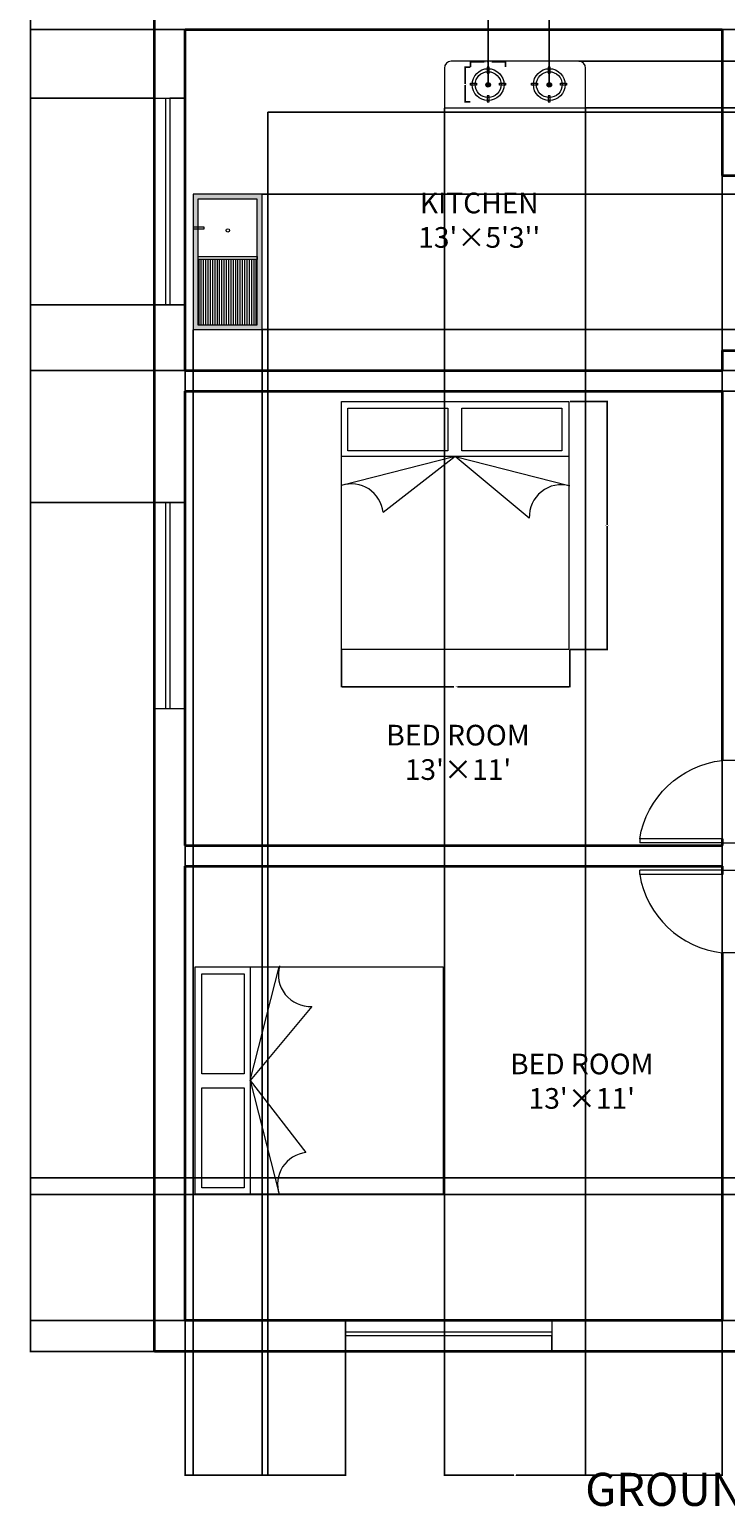
# Model space of a CAD drawing. Units: inches. Extents: x 1108 to 1543, y 442 to 1097.
# Tile 1 of 3: x 1108 to 1310, y 442 to 871. Entities that reach past the tile are written whole.
import ezdxf

# ---------------------------------------------------------------- set-up
doc = ezdxf.new("R2010")
doc.units = ezdxf.units.IN
for name, color, linetype, lineweight in [('A-ANNO-DIMS', 2, 'Continuous', 18), ('A-ANNO-TEXT', 7, 'Continuous', 25), ('A-AREA-IDEN', 7, 'Continuous', 18), ('A-DOOR', 4, 'Continuous', 18), ('A-EQPM', 8, 'Continuous', 18), ('A-FLOR-CASE', 8, 'Continuous', 25), ('A-FLOR-FIXT', 9, 'Continuous', 18), ('A-FLOR-FIXT-PATT', 9, 'Continuous', 13), ('A-FURN', 8, 'Continuous', 18), ('A-GLAZ', 5, 'Continuous', 18), ('A-WALL', 7, 'Continuous', 35)]:
    doc.layers.add(name, color=color, linetype=linetype, lineweight=lineweight)
doc.styles.get("Standard").update_dxf_attribs({"font": 'times.ttf'})
doc.dimstyles.get("Standard").update_dxf_attribs({"dimtxt": 0.18, "dimasz": 0.18, "dimexe": 0.18, "dimexo": 0.0625, "dimgap": 0.09, "dimtad": 0, "dimtih": 1, "dimtoh": 1, "dimdec": 4, "dimzin": 0, "dimdsep": 46, "dimtxsty": 'Standard', "dimcen": 0.09, "dimadec": 0, "dimazin": 0, "dimtfac": 1, "dimtdec": 4, "dimtofl": 0, "dimtmove": 0, "dimatfit": 3, "dimfxl": 1, "dimtolj": 1, "dimtzin": 0, "dimarcsym": 0})

# ---------------------------------------------------------------- blocks, each defined once
blk = doc.blocks.new('d')
for p, q in [((1309.33, 626.48), (1285.33, 626.48)), ((1285.33, 625.28), (1285.33, 626.48)), ((1309.33, 626.48), (1315.33, 626.48)), ((1309.33, 625.28), (1285.33, 625.28)), ((1315.33, 602.48), (1309.33, 602.48))]:
    blk.add_line(p, q)
blk.add_arc((1312.52, 629.86), 27.57, 189.5705, 263.3671)
blk = doc.blocks.new('BED-DOUBLE-66X72')
for p, q in [((0, 0), (0, 72)), ((0, 72), (66, 72)), ((66, 72), (66, 0)), ((66, 56.1), (0, 56.1)), ((33, 56.1), (0, 47.62)), ((33, 56.1), (12.08, 39.84)), ((33, 56.1), (66, 47.62)), ((54.54, 38.14), (33, 56.1)), ((66, 0), (0, 0))]:
    blk.add_line(p, q)
for points in [[(30.92, 70.13), (30.92, 57.75), (1.83, 57.75), (1.83, 70.13)], [(64.01, 70.13), (64.01, 57.75), (34.92, 57.75), (34.92, 70.13)]]:
    blk.add_lwpolyline(points, close=True)
for centre, radius, start, end in [((2.92, 38.89), 9.21, 5.9499, 108.4921), ((63.85, 38.55), 9.32, 74.4856, 182.5542)]:
    blk.add_arc(centre, radius, start, end)
blk = doc.blocks.new('WIN-60IN')
for p, q in [((-9, -60), (-9, 0)), ((-9, 0), (0, 0)), ((-5.7, -60), (-5.7, 0)), ((0, 0), (-4.5, 0)), ((-4.5, 0), (-4.5, -60)), ((0, 0), (0, -60)), ((0, -60), (-9, -60)), ((-4.5, -60), (-5.7, -60))]:
    blk.add_line(p, q)
blk = doc.blocks.new('HOB-BURNER')
h = blk.add_hatch(color=256)
h.dxf.hatch_style = 1
h.paths.add_polyline_path([(0.67, -0.05, 1), (-0.65, -0.05, 1)])
for points in [[(-0.28, 3.35), (0.3, 3.35), (0.3, 5.06), (-0.28, 5.06)], [(-5.14, 0.42), (-3.39, 0.42), (-3.39, -0.14), (-5.14, -0.14)], [(3.29, 0.42), (5.04, 0.42), (5.04, -0.14), (3.29, -0.14)], [(-0.28, -5), (0.3, -5), (0.3, -3.29), (-0.28, -3.29)]]:
    blk.add_lwpolyline(points, close=True)
for centre, radius in [((0, 0), 4.63), ((0, 0), 3.76), ((0.01, -0.05), 0.661)]:
    blk.add_circle(centre, radius)
blk = doc.blocks.new('*D11')
at = {"layer": 'A-ANNO-DIMS', "color": 0, "lineweight": -2, "transparency": 16777216}
for p, q in [((1265.13, 762.59), (1276.05, 762.59)), ((1275.87, 762.41), (1275.87, 726.77)), ((1275.87, 690.77), (1275.87, 726.41)), ((1265.13, 690.59), (1276.05, 690.59))]:
    blk.add_line(p, q, dxfattribs=at)
at = {"layer": 'A-ANNO-DIMS', "color": 0, "transparency": 16777216}
for points in [[(1275.84, 762.41), (1275.9, 762.41), (1275.87, 762.59)], [(1275.84, 690.77), (1275.9, 690.77), (1275.87, 690.59)]]:
    blk.add_solid(points, dxfattribs=at)
at = {"layer": 'Defpoints', "color": 0, "transparency": 16777216}
for p in [(1265.07, 762.59), (1275.87, 762.59), (1265.07, 690.59)]:
    blk.add_point(p, dxfattribs=at)
at = {"layer": 'A-ANNO-DIMS', "color": 0, "transparency": 16777216, "insert": (1275.87, 726.59), "char_height": 0.18, "attachment_point": 5}
blk.add_mtext('\\A1;BED 72 TYP.', dxfattribs=at)
blk = doc.blocks.new('*D12')
at = {"layer": 'A-ANNO-DIMS', "color": 0, "lineweight": -2, "transparency": 16777216}
for p, q in [((1198.72, 690.53), (1198.72, 679.61)), ((1265.07, 690.53), (1265.07, 679.61)), ((1198.9, 679.79), (1231.37, 679.79)), ((1264.89, 679.79), (1232.42, 679.79))]:
    blk.add_line(p, q, dxfattribs=at)
at = {"layer": 'A-ANNO-DIMS', "color": 0, "transparency": 16777216}
for points in [[(1198.9, 679.82), (1198.9, 679.76), (1198.72, 679.79)], [(1264.89, 679.82), (1264.89, 679.76), (1265.07, 679.79)]]:
    blk.add_solid(points, dxfattribs=at)
at = {"layer": 'Defpoints', "color": 0, "transparency": 16777216}
for p in [(1198.72, 690.59), (1265.07, 690.59), (1265.07, 679.79)]:
    blk.add_point(p, dxfattribs=at)
at = {"layer": 'A-ANNO-DIMS', "color": 0, "transparency": 16777216, "insert": (1231.89, 679.79), "char_height": 0.18, "attachment_point": 5}
blk.add_mtext('\\A1;66 TYP.', dxfattribs=at)
blk = doc.blocks.new('*D13')
at = {"layer": 'A-ANNO-DIMS', "color": 0, "lineweight": -2, "transparency": 16777216}
for p, q in [((1236.15, 859.8), (1236.15, 861.45)), ((1236.33, 861.27), (1240.14, 861.27)), ((1246.15, 861.27), (1242.34, 861.27)), ((1246.33, 859.8), (1246.33, 861.45))]:
    blk.add_line(p, q, dxfattribs=at)
at = {"layer": 'A-ANNO-DIMS', "color": 0, "transparency": 16777216}
for points in [[(1236.33, 861.3), (1236.33, 861.24), (1236.15, 861.27)], [(1246.15, 861.3), (1246.15, 861.24), (1246.33, 861.27)]]:
    blk.add_solid(points, dxfattribs=at)
at = {"layer": 'Defpoints', "color": 0, "transparency": 16777216}
for p in [(1236.15, 859.74), (1246.33, 861.27), (1246.33, 859.74)]:
    blk.add_point(p, dxfattribs=at)
at = {"layer": 'A-ANNO-DIMS', "color": 0, "transparency": 16777216, "insert": (1241.24, 861.27), "char_height": 0.18, "attachment_point": 5}
blk.add_mtext('\\A1;BURNER 10 TYP.', dxfattribs=at)
blk = doc.blocks.new('*D14')
at = {"layer": 'A-ANNO-DIMS', "color": 0, "lineweight": -2, "transparency": 16777216}
for p, q in [((1236.09, 859.74), (1234.44, 859.74)), ((1234.62, 859.56), (1234.62, 854.89)), ((1234.62, 849.86), (1234.62, 854.53)), ((1236.09, 849.68), (1234.44, 849.68))]:
    blk.add_line(p, q, dxfattribs=at)
at = {"layer": 'A-ANNO-DIMS', "color": 0, "transparency": 16777216}
for points in [[(1234.59, 859.56), (1234.65, 859.56), (1234.62, 859.74)], [(1234.59, 849.86), (1234.65, 849.86), (1234.62, 849.68)]]:
    blk.add_solid(points, dxfattribs=at)
at = {"layer": 'Defpoints', "color": 0, "transparency": 16777216}
for p in [(1234.62, 859.74), (1236.15, 859.74), (1236.15, 849.68)]:
    blk.add_point(p, dxfattribs=at)
at = {"layer": 'A-ANNO-DIMS', "color": 0, "transparency": 16777216, "insert": (1234.62, 854.71), "char_height": 0.18, "attachment_point": 5}
blk.add_mtext('\\A1;10 TYP.', dxfattribs=at)
blk = doc.blocks.new('*D16')
at = {"layer": 'A-ANNO-DIMS', "color": 0, "lineweight": -2, "transparency": 16777216}
for p, q in [((1144.27, 1029.68), (1108.2, 1029.68)), ((1108.38, 1029.5), (1108.38, 758.36)), ((1108.38, 486.86), (1108.38, 758)), ((1144.27, 486.68), (1108.2, 486.68))]:
    blk.add_line(p, q, dxfattribs=at)
at = {"layer": 'A-ANNO-DIMS', "color": 0, "transparency": 16777216}
for points in [[(1108.35, 1029.5), (1108.41, 1029.5), (1108.38, 1029.68)], [(1108.35, 486.86), (1108.41, 486.86), (1108.38, 486.68)]]:
    blk.add_solid(points, dxfattribs=at)
at = {"layer": 'Defpoints', "color": 0, "transparency": 16777216}
for p in [(1108.38, 1029.68), (1144.33, 1029.68), (1144.33, 486.68)]:
    blk.add_point(p, dxfattribs=at)
at = {"layer": 'A-ANNO-DIMS', "color": 0, "transparency": 16777216, "insert": (1108.38, 758.18), "char_height": 0.18, "attachment_point": 5}
blk.add_mtext('\\A1;543', dxfattribs=at)
blk = doc.blocks.new('*D18')
at = {"layer": 'A-ANNO-DIMS', "color": 0, "lineweight": -2, "transparency": 16777216}
for p, q in [((1144.27, 915.48), (1108.2, 915.48)), ((1108.38, 915.3), (1108.38, 883.28)), ((1108.38, 850.9), (1108.38, 882.92)), ((1144.27, 850.72), (1108.2, 850.72))]:
    blk.add_line(p, q, dxfattribs=at)
at = {"layer": 'A-ANNO-DIMS', "color": 0, "transparency": 16777216}
for points in [[(1108.35, 915.3), (1108.41, 915.3), (1108.38, 915.48)], [(1108.35, 850.9), (1108.41, 850.9), (1108.38, 850.72)]]:
    blk.add_solid(points, dxfattribs=at)
at = {"layer": 'Defpoints', "color": 0, "transparency": 16777216}
for p in [(1144.33, 915.48), (1108.38, 850.72), (1144.33, 850.72)]:
    blk.add_point(p, dxfattribs=at)
at = {"layer": 'A-ANNO-DIMS', "color": 0, "transparency": 16777216, "insert": (1108.38, 883.1), "char_height": 0.18, "attachment_point": 5}
blk.add_mtext('\\A1;64.76', dxfattribs=at)
blk = doc.blocks.new('*D19')
at = {"layer": 'A-ANNO-DIMS', "color": 0, "lineweight": -2, "transparency": 16777216}
for p, q in [((1153.27, 790.72), (1108.2, 790.72)), ((1108.38, 790.54), (1108.38, 762.2)), ((1108.38, 733.49), (1108.38, 761.83)), ((1153.27, 733.31), (1108.2, 733.31))]:
    blk.add_line(p, q, dxfattribs=at)
at = {"layer": 'A-ANNO-DIMS', "color": 0, "transparency": 16777216}
for points in [[(1108.35, 790.54), (1108.41, 790.54), (1108.38, 790.72)], [(1108.35, 733.49), (1108.41, 733.49), (1108.38, 733.31)]]:
    blk.add_solid(points, dxfattribs=at)
at = {"layer": 'Defpoints', "color": 0, "transparency": 16777216}
for p in [(1153.33, 790.72), (1108.38, 733.31), (1153.33, 733.31)]:
    blk.add_point(p, dxfattribs=at)
at = {"layer": 'A-ANNO-DIMS', "color": 0, "transparency": 16777216, "insert": (1108.38, 762.02), "char_height": 0.18, "attachment_point": 5}
blk.add_mtext('\\A1;57.4', dxfattribs=at)
blk = doc.blocks.new('*D25')
at = {"layer": 'A-ANNO-DIMS', "color": 0, "lineweight": -2, "transparency": 16777216}
for p, q in [((1153.33, 495.62), (1153.33, 450.55)), ((1199.83, 495.62), (1199.83, 450.55)), ((1153.51, 450.73), (1176.27, 450.73)), ((1199.65, 450.73), (1176.9, 450.73))]:
    blk.add_line(p, q, dxfattribs=at)
at = {"layer": 'A-ANNO-DIMS', "color": 0, "transparency": 16777216}
for points in [[(1153.51, 450.76), (1153.51, 450.7), (1153.33, 450.73)], [(1199.65, 450.76), (1199.65, 450.7), (1199.83, 450.73)]]:
    blk.add_solid(points, dxfattribs=at)
at = {"layer": 'Defpoints', "color": 0, "transparency": 16777216}
for p in [(1153.33, 495.68), (1199.83, 495.68), (1199.83, 450.73)]:
    blk.add_point(p, dxfattribs=at)
at = {"layer": 'A-ANNO-DIMS', "color": 0, "transparency": 16777216, "insert": (1176.58, 450.73), "char_height": 0.18, "attachment_point": 5}
blk.add_mtext('\\A1;46.5', dxfattribs=at)
blk = doc.blocks.new('*D36')
at = {"layer": 'A-ANNO-DIMS', "color": 0, "lineweight": -2, "transparency": 16777216}
for p, q in [((1381.27, 532.28), (1108.2, 532.28)), ((1108.38, 532.1), (1108.38, 514.16)), ((1108.38, 495.86), (1108.38, 513.8)), ((1381.27, 495.68), (1108.2, 495.68))]:
    blk.add_line(p, q, dxfattribs=at)
at = {"layer": 'A-ANNO-DIMS', "color": 0, "transparency": 16777216}
for points in [[(1108.35, 532.1), (1108.41, 532.1), (1108.38, 532.28)], [(1108.35, 495.86), (1108.41, 495.86), (1108.38, 495.68)]]:
    blk.add_solid(points, dxfattribs=at)
at = {"layer": 'Defpoints', "color": 0, "transparency": 16777216}
for p in [(1381.33, 532.28), (1108.38, 495.68), (1381.33, 495.68)]:
    blk.add_point(p, dxfattribs=at)
at = {"layer": 'A-ANNO-DIMS', "color": 0, "transparency": 16777216, "insert": (1108.38, 513.98), "char_height": 0.18, "attachment_point": 5}
blk.add_mtext('\\A1;36.6', dxfattribs=at)
blk = doc.blocks.new('*D37')
at = {"layer": 'A-ANNO-DIMS', "color": 0, "lineweight": -2, "transparency": 16777216}
for p, q in [((1309.4, 771.68), (1542.46, 771.68)), ((1542.28, 771.5), (1542.28, 768.86)), ((1542.28, 765.86), (1542.28, 768.5)), ((1309.4, 765.68), (1542.46, 765.68))]:
    blk.add_line(p, q, dxfattribs=at)
at = {"layer": 'A-ANNO-DIMS', "color": 0, "transparency": 16777216}
for points in [[(1542.25, 771.5), (1542.31, 771.5), (1542.28, 771.68)], [(1542.25, 765.86), (1542.31, 765.86), (1542.28, 765.68)]]:
    blk.add_solid(points, dxfattribs=at)
at = {"layer": 'Defpoints', "color": 0, "transparency": 16777216}
for p in [(1309.33, 771.68), (1542.28, 771.68), (1309.33, 765.68)]:
    blk.add_point(p, dxfattribs=at)
at = {"layer": 'A-ANNO-DIMS', "color": 0, "transparency": 16777216, "insert": (1542.28, 768.68), "char_height": 0.18, "attachment_point": 5}
blk.add_mtext('\\A1;6', dxfattribs=at)
blk = doc.blocks.new('*D38')
at = {"layer": 'A-ANNO-DIMS', "color": 0, "lineweight": -2, "transparency": 16777216}
for p, q in [((1153.27, 870.68), (1108.2, 870.68)), ((1108.38, 870.5), (1108.38, 821.36)), ((1108.38, 771.86), (1108.38, 821)), ((1153.27, 771.68), (1108.2, 771.68))]:
    blk.add_line(p, q, dxfattribs=at)
at = {"layer": 'A-ANNO-DIMS', "color": 0, "transparency": 16777216}
for points in [[(1108.35, 870.5), (1108.41, 870.5), (1108.38, 870.68)], [(1108.35, 771.86), (1108.41, 771.86), (1108.38, 771.68)]]:
    blk.add_solid(points, dxfattribs=at)
at = {"layer": 'Defpoints', "color": 0, "transparency": 16777216}
for p in [(1108.38, 870.68), (1153.33, 870.68), (1153.33, 771.68)]:
    blk.add_point(p, dxfattribs=at)
at = {"layer": 'A-ANNO-DIMS', "color": 0, "transparency": 16777216, "insert": (1108.38, 821.18), "char_height": 0.18, "attachment_point": 5}
blk.add_mtext('\\A1;99', dxfattribs=at)
blk = doc.blocks.new('*D40')
at = {"layer": 'A-ANNO-DIMS', "color": 0, "lineweight": -2, "transparency": 16777216}
for p, q in [((1153.33, 771.62), (1153.33, 450.55)), ((1177.33, 771.62), (1177.33, 450.55)), ((1153.51, 450.73), (1165.12, 450.73)), ((1177.15, 450.73), (1165.55, 450.73))]:
    blk.add_line(p, q, dxfattribs=at)
at = {"layer": 'A-ANNO-DIMS', "color": 0, "transparency": 16777216}
for points in [[(1153.51, 450.76), (1153.51, 450.7), (1153.33, 450.73)], [(1177.15, 450.76), (1177.15, 450.7), (1177.33, 450.73)]]:
    blk.add_solid(points, dxfattribs=at)
at = {"layer": 'Defpoints', "color": 0, "transparency": 16777216}
for p in [(1153.33, 771.68), (1177.33, 771.68), (1177.33, 450.73)]:
    blk.add_point(p, dxfattribs=at)
at = {"layer": 'A-ANNO-DIMS', "color": 0, "transparency": 16777216, "insert": (1165.33, 450.73), "char_height": 0.18, "attachment_point": 5}
blk.add_mtext('\\A1;24', dxfattribs=at)
blk = doc.blocks.new('*D41')
at = {"layer": 'A-ANNO-DIMS', "color": 0, "lineweight": -2, "transparency": 16777216}
for p, q in [((1155.62, 783.47), (1155.62, 450.55)), ((1175.65, 783.47), (1175.65, 450.55)), ((1155.8, 450.73), (1165.19, 450.73)), ((1175.47, 450.73), (1166.08, 450.73))]:
    blk.add_line(p, q, dxfattribs=at)
at = {"layer": 'A-ANNO-DIMS', "color": 0, "transparency": 16777216}
for points in [[(1155.8, 450.76), (1155.8, 450.7), (1155.62, 450.73)], [(1175.47, 450.76), (1175.47, 450.7), (1175.65, 450.73)]]:
    blk.add_solid(points, dxfattribs=at)
at = {"layer": 'Defpoints', "color": 0, "transparency": 16777216}
for p in [(1155.62, 783.54), (1175.65, 783.54), (1175.65, 450.73)]:
    blk.add_point(p, dxfattribs=at)
at = {"layer": 'A-ANNO-DIMS', "color": 0, "transparency": 16777216, "insert": (1165.64, 450.73), "char_height": 0.18, "attachment_point": 5}
blk.add_mtext('\\A1;20.035', dxfattribs=at)
blk = doc.blocks.new('*D42')
at = {"layer": 'A-ANNO-DIMS', "color": 0, "lineweight": -2, "transparency": 16777216}
for p, q in [((1175.72, 822.87), (1542.46, 822.87)), ((1542.28, 822.69), (1542.28, 803.38)), ((1542.28, 783.72), (1542.28, 803.02)), ((1175.72, 783.54), (1542.46, 783.54))]:
    blk.add_line(p, q, dxfattribs=at)
at = {"layer": 'A-ANNO-DIMS', "color": 0, "transparency": 16777216}
for points in [[(1542.25, 822.69), (1542.31, 822.69), (1542.28, 822.87)], [(1542.25, 783.72), (1542.31, 783.72), (1542.28, 783.54)]]:
    blk.add_solid(points, dxfattribs=at)
at = {"layer": 'Defpoints', "color": 0, "transparency": 16777216}
for p in [(1175.65, 822.87), (1542.28, 822.87), (1175.65, 783.54)]:
    blk.add_point(p, dxfattribs=at)
at = {"layer": 'A-ANNO-DIMS', "color": 0, "transparency": 16777216, "insert": (1542.28, 803.2), "char_height": 0.18, "attachment_point": 5}
blk.add_mtext('\\A1;39.33', dxfattribs=at)
blk = doc.blocks.new('*D43')
at = {"layer": 'A-ANNO-DIMS', "color": 0, "lineweight": -2, "transparency": 16777216}
for p, q in [((1175.72, 783.54), (1542.46, 783.54)), ((1542.28, 783.36), (1542.28, 777.79)), ((1542.28, 771.86), (1542.28, 777.43)), ((1177.4, 771.68), (1542.46, 771.68))]:
    blk.add_line(p, q, dxfattribs=at)
at = {"layer": 'A-ANNO-DIMS', "color": 0, "transparency": 16777216}
for points in [[(1542.25, 783.36), (1542.31, 783.36), (1542.28, 783.54)], [(1542.25, 771.86), (1542.31, 771.86), (1542.28, 771.68)]]:
    blk.add_solid(points, dxfattribs=at)
at = {"layer": 'Defpoints', "color": 0, "transparency": 16777216}
for p in [(1175.65, 783.54), (1177.33, 771.68), (1542.28, 771.68)]:
    blk.add_point(p, dxfattribs=at)
at = {"layer": 'A-ANNO-DIMS', "color": 0, "transparency": 16777216, "insert": (1542.28, 777.61), "char_height": 0.18, "attachment_point": 5}
blk.add_mtext('\\A1;11.857', dxfattribs=at)
blk = doc.blocks.new('*D44')
at = {"layer": 'A-ANNO-DIMS', "color": 0, "lineweight": -2, "transparency": 16777216}
for p, q in [((1228.6, 847.87), (1228.6, 450.55)), ((1269.61, 847.87), (1269.61, 450.55)), ((1228.78, 450.73), (1248.73, 450.73)), ((1269.43, 450.73), (1249.48, 450.73))]:
    blk.add_line(p, q, dxfattribs=at)
at = {"layer": 'A-ANNO-DIMS', "color": 0, "transparency": 16777216}
for points in [[(1228.78, 450.76), (1228.78, 450.7), (1228.6, 450.73)], [(1269.43, 450.76), (1269.43, 450.7), (1269.61, 450.73)]]:
    blk.add_solid(points, dxfattribs=at)
at = {"layer": 'Defpoints', "color": 0, "transparency": 16777216}
for p in [(1228.6, 847.93), (1269.61, 847.93), (1269.61, 450.73)]:
    blk.add_point(p, dxfattribs=at)
at = {"layer": 'A-ANNO-DIMS', "color": 0, "transparency": 16777216, "insert": (1249.1, 450.73), "char_height": 0.18, "attachment_point": 5}
blk.add_mtext('\\A1;41.01', dxfattribs=at)
blk = doc.blocks.new('*D45')
at = {"layer": 'A-ANNO-DIMS', "color": 0, "lineweight": -2, "transparency": 16777216}
for p, q in [((1269.61, 847.87), (1269.61, 450.55)), ((1309.33, 846.62), (1309.33, 450.55)), ((1269.79, 450.73), (1289.1, 450.73)), ((1309.15, 450.73), (1289.84, 450.73))]:
    blk.add_line(p, q, dxfattribs=at)
at = {"layer": 'A-ANNO-DIMS', "color": 0, "transparency": 16777216}
for points in [[(1269.79, 450.76), (1269.79, 450.7), (1269.61, 450.73)], [(1309.15, 450.76), (1309.15, 450.7), (1309.33, 450.73)]]:
    blk.add_solid(points, dxfattribs=at)
at = {"layer": 'Defpoints', "color": 0, "transparency": 16777216}
for p in [(1269.61, 847.93), (1309.33, 846.68), (1309.33, 450.73)]:
    blk.add_point(p, dxfattribs=at)
at = {"layer": 'A-ANNO-DIMS', "color": 0, "transparency": 16777216, "insert": (1289.47, 450.73), "char_height": 0.18, "attachment_point": 5}
blk.add_mtext('\\A1;39.73', dxfattribs=at)
blk = doc.blocks.new('*D46')
at = {"layer": 'A-ANNO-DIMS', "color": 0, "lineweight": -2, "transparency": 16777216}
for p, q in [((1309.397156, 870.679098), (1542.464656, 870.679098)), ((1542.284656, 870.499098), (1542.284656, 858.859098)), ((1542.284656, 846.859098), (1542.284656, 858.499098)), ((1309.397156, 846.679098), (1542.464656, 846.679098))]:
    blk.add_line(p, q, dxfattribs=at)
at = {"layer": 'A-ANNO-DIMS', "color": 0, "transparency": 16777216}
for points in [[(1542.254656, 870.499098), (1542.314656, 870.499098), (1542.284656, 870.679098)], [(1542.254656, 846.859098), (1542.314656, 846.859098), (1542.284656, 846.679098)]]:
    blk.add_solid(points, dxfattribs=at)
at = {"layer": 'Defpoints', "color": 0, "transparency": 16777216}
for p in [(1309.334656, 870.679098), (1542.284656, 870.679098), (1309.334656, 846.679098)]:
    blk.add_point(p, dxfattribs=at)
at = {"layer": 'A-ANNO-DIMS', "color": 0, "transparency": 16777216, "insert": (1542.284656, 858.679098), "char_height": 0.18, "attachment_point": 5}
blk.add_mtext('\\A1;24', dxfattribs=at)
blk = doc.blocks.new('*D47')
at = {"layer": 'A-ANNO-DIMS', "color": 0, "lineweight": -2, "transparency": 16777216}
for p, q in [((1309.4, 846.68), (1542.46, 846.68)), ((1542.28, 846.5), (1542.28, 837.67)), ((1542.28, 828.47), (1542.28, 837.3)), ((1309.4, 828.29), (1542.46, 828.29))]:
    blk.add_line(p, q, dxfattribs=at)
at = {"layer": 'A-ANNO-DIMS', "color": 0, "transparency": 16777216}
for points in [[(1542.25, 846.5), (1542.31, 846.5), (1542.28, 846.68)], [(1542.25, 828.47), (1542.31, 828.47), (1542.28, 828.29)]]:
    blk.add_solid(points, dxfattribs=at)
at = {"layer": 'Defpoints', "color": 0, "transparency": 16777216}
for p in [(1309.33, 846.68), (1542.28, 846.68), (1309.33, 828.29)]:
    blk.add_point(p, dxfattribs=at)
at = {"layer": 'A-ANNO-DIMS', "color": 0, "transparency": 16777216, "insert": (1542.28, 837.48), "char_height": 0.18, "attachment_point": 5}
blk.add_mtext('\\A1;18.39', dxfattribs=at)
blk = doc.blocks.new('*D48')
at = {"layer": 'A-ANNO-DIMS', "color": 0, "lineweight": -2, "transparency": 16777216}
for p, q in [((1267.67, 861.48), (1542.46, 861.48)), ((1542.28, 861.3), (1542.28, 854.89)), ((1542.28, 848.11), (1542.28, 854.52)), ((1269.67, 847.93), (1542.46, 847.93))]:
    blk.add_line(p, q, dxfattribs=at)
at = {"layer": 'A-ANNO-DIMS', "color": 0, "transparency": 16777216}
for points in [[(1542.25, 861.3), (1542.31, 861.3), (1542.28, 861.48)], [(1542.25, 848.11), (1542.31, 848.11), (1542.28, 847.93)]]:
    blk.add_solid(points, dxfattribs=at)
at = {"layer": 'Defpoints', "color": 0, "transparency": 16777216}
for p in [(1267.61, 861.48), (1542.28, 861.48), (1269.61, 847.93)]:
    blk.add_point(p, dxfattribs=at)
at = {"layer": 'A-ANNO-DIMS', "color": 0, "transparency": 16777216, "insert": (1542.28, 854.71), "char_height": 0.18, "attachment_point": 5}
blk.add_mtext('\\A1;13.556', dxfattribs=at)
blk = doc.blocks.new('*D49')
at = {"layer": 'A-ANNO-DIMS', "color": 0, "lineweight": -2, "transparency": 16777216}
for p, q in [((1241.29, 854.74), (1241.29, 1097.43)), ((1241.47, 1097.25), (1249.81, 1097.25)), ((1258.89, 1097.25), (1250.55, 1097.25)), ((1259.07, 854.74), (1259.07, 1097.43))]:
    blk.add_line(p, q, dxfattribs=at)
at = {"layer": 'A-ANNO-DIMS', "color": 0, "transparency": 16777216}
for points in [[(1241.47, 1097.28), (1241.47, 1097.22), (1241.29, 1097.25)], [(1258.89, 1097.28), (1258.89, 1097.22), (1259.07, 1097.25)]]:
    blk.add_solid(points, dxfattribs=at)
at = {"layer": 'Defpoints', "color": 0, "transparency": 16777216}
for p in [(1259.07, 1097.25), (1241.29, 854.68), (1259.07, 854.68)]:
    blk.add_point(p, dxfattribs=at)
at = {"layer": 'A-ANNO-DIMS', "color": 0, "transparency": 16777216, "insert": (1250.18, 1097.25), "char_height": 0.18, "attachment_point": 5}
blk.add_mtext('\\A1;17.78', dxfattribs=at)
blk = doc.blocks.new('*D51')
at = {"layer": 'A-ANNO-DIMS', "color": 0, "lineweight": -2, "transparency": 16777216}
for p, q in [((1381.27, 537.08), (1108.2, 537.08)), ((1108.38, 536.9), (1108.38, 534.86)), ((1381.27, 532.28), (1108.2, 532.28)), ((1108.38, 532.46), (1108.38, 534.5))]:
    blk.add_line(p, q, dxfattribs=at)
at = {"layer": 'A-ANNO-DIMS', "color": 0, "transparency": 16777216}
for points in [[(1108.35, 536.9), (1108.41, 536.9), (1108.38, 537.08)], [(1108.35, 532.46), (1108.41, 532.46), (1108.38, 532.28)]]:
    blk.add_solid(points, dxfattribs=at)
at = {"layer": 'Defpoints', "color": 0, "transparency": 16777216}
for p in [(1381.33, 537.08), (1108.38, 532.28), (1381.33, 532.28)]:
    blk.add_point(p, dxfattribs=at)
at = {"layer": 'A-ANNO-DIMS', "color": 0, "transparency": 16777216, "insert": (1108.38, 534.68), "char_height": 0.18, "attachment_point": 5}
blk.add_mtext('\\A1;4.8', dxfattribs=at)

msp = doc.modelspace()

# ---------------------------------------------------------------- hatches: boundary and pattern name
at = {"layer": 'A-FLOR-FIXT-PATT'}
h = msp.add_hatch(color=256, dxfattribs=at)
h.dxf.hatch_style = 1
h.paths.add_polyline_path([(1175.6532, 822.8655), (1155.6177, 822.8655), (1155.6177, 813.4162), (1156.9399, 813.4162), (1156.9399, 821.4208), (1174.2531, 821.4208), (1174.2531, 784.878), (1156.9399, 784.878), (1156.9399, 812.6705), (1155.6177, 812.6705), (1155.6177, 783.5357), (1175.6532, 783.5357)])
h.paths.add_polyline_path([(1156.9399, 813.4162), (1155.6177, 813.4162), (1155.6177, 812.6705), (1156.9399, 812.6705)], flags=17)
h = msp.add_hatch(dxfattribs=at)
h.set_pattern_fill('ANSI31', color=256, scale=0.2097292, angle=45, style=0)
h.paths.add_polyline_path([(1156.9399, 784.878), (1174.2531, 784.878), (1174.2531, 803.9201), (1156.9399, 803.9201)])

# ---------------------------------------------------------------- linework, layer by layer
at = {"layer": 'A-DOOR'}
for p, q in [((1309.3347, 635.5864), (1309.3347, 634.3864)), ((1309.3347, 626.4791), (1309.3347, 625.2791)), ((1309.3347, 625.2791), (1309.3347, 626.4791))]:
    msp.add_line(p, q, dxfattribs=at)
at = {"layer": 'A-EQPM'}
msp.add_lwpolyline([(1228.6012, 847.9289), (1269.6075, 847.9289), (1269.6075, 859.4845, 0.41421356), (1267.6075, 861.4845), (1230.6012, 861.4845, 0.41421356), (1228.6012, 859.4845)], format="xyb", close=True, dxfattribs=at)
at = {"layer": 'A-FLOR-CASE'}
for p, q in [((1309.3347, 870.6791), (1309.3347, 846.6791)), ((1309.3347, 846.6791), (1177.3347, 846.6791)), ((1177.3347, 846.6791), (1177.3347, 771.6791))]:
    msp.add_line(p, q, dxfattribs=at)
at = {"layer": 'A-FLOR-FIXT'}
for p, q in [((1155.6177, 813.4162), (1158.6812, 813.4162)), ((1158.6812, 812.6705), (1155.6177, 812.6705)), ((1158.6812, 813.4162), (1158.6812, 812.6705)), ((1156.9399, 804.7156), (1174.2531, 804.7156)), ((1174.2531, 803.9201), (1156.9399, 803.9201)), ((1174.2531, 804.7156), (1174.2531, 803.9201))]:
    msp.add_line(p, q, dxfattribs=at)
for points in [[(1155.6177, 783.5357), (1175.6532, 783.5357), (1175.6532, 822.8655), (1155.6177, 822.8655)], [(1156.9399, 784.878), (1174.2531, 784.878), (1174.2531, 821.4208), (1156.9399, 821.4208)]]:
    msp.add_lwpolyline(points, close=True, dxfattribs=at)
msp.add_circle((1165.696, 812.3224), 0.4975, dxfattribs=at)
at = {"layer": 'A-WALL'}
for p, q in [((1144.3347, 486.6791), (1144.3347, 1029.6791)), ((1153.3347, 771.6791), (1153.3347, 870.6791)), ((1153.3347, 870.6791), (1309.3347, 870.6791)), ((1309.3347, 870.6791), (1309.3347, 828.2882)), ((1309.3347, 828.2882), (1315.3347, 828.2882)), ((1309.3347, 777.4792), (1315.3347, 777.4792)), ((1309.3347, 777.4792), (1309.3347, 771.6791)), ((1153.3347, 771.6791), (1309.3347, 771.6791)), ((1153.3347, 633.6791), (1153.3347, 765.6791)), ((1153.3347, 765.6791), (1309.3347, 765.6791)), ((1309.3347, 765.6791), (1309.3347, 658.3864)), ((1309.3347, 635.5864), (1309.3347, 633.6791)), ((1153.3347, 633.6791), (1309.3347, 633.6791)), ((1153.3347, 495.6791), (1153.3347, 627.6791)), ((1153.3347, 627.6791), (1309.3347, 627.6791)), ((1309.3347, 627.6791), (1309.3347, 625.2791)), ((1309.3347, 627.6791), (1309.3347, 626.4791)), ((1309.3347, 602.4791), (1309.3347, 495.6791)), ((1309.3347, 495.6791), (1153.3347, 495.6791)), ((1315.3347, 486.6791), (1144.3347, 486.6791))]:
    msp.add_line(p, q, dxfattribs=at)

# ---------------------------------------------------------------- block references
at = {"layer": 'A-DOOR', "xscale": -1, "rotation": 180}
msp.add_blockref('d', (0, 1260.8655), dxfattribs=at)
at = {"layer": 'A-DOOR'}
msp.add_blockref('d', (0, 0), dxfattribs=at)
at = {"layer": 'A-EQPM'}
for p in [(1241.2895, 854.6808), (1259.07, 854.6808)]:
    msp.add_blockref('HOB-BURNER', p, dxfattribs=at)
at = {"layer": 'A-FURN'}
msp.add_blockref('BED-DOUBLE-66X72', (1198.7207, 690.5931), dxfattribs=at)
at = {"layer": 'A-FURN', "rotation": 89.99999999999984}
msp.add_blockref('BED-DOUBLE-66X72', (1228.2273, 532.3704), dxfattribs=at)
at = {"layer": 'A-GLAZ'}
for p in [(1153.3347, 850.719), (1153.3347, 733.3139)]:
    msp.add_blockref('WIN-60IN', p, dxfattribs=at)
at = {"layer": 'A-GLAZ', "rotation": 269.9999999999998}
msp.add_blockref('WIN-60IN', (1259.8347, 486.6791), dxfattribs=at)

# ---------------------------------------------------------------- texts
at = {"layer": 'A-ANNO-TEXT', "insert": (1202.8439, 451.4335), "char_height": 9.6, "attachment_point": 1}
msp.add_mtext_dynamic_manual_height_columns('\\pxqc;GROUND FLOOR PLAN', width=269.09847, gutter_width=12.5, heights=[0], dxfattribs=at)
at = {"layer": 'A-AREA-IDEN', "char_height": 6, "attachment_point": 1}
for s, insert in [("\\pxqc;KITCHEN\\P13'×5'3''", (1104.1699, 823.2923)), ("\\pxqc;BED ROOM\\P13'×11'", (1098.0033, 668.7147)), ("\\pxqc;BED ROOM\\P13'×11'", (1133.975, 573.1951))]:
    msp.add_mtext_dynamic_manual_height_columns(s, width=269.09847, gutter_width=12.5, heights=[0], dxfattribs=dict(at, insert=insert))

# ---------------------------------------------------------------- dimensions: what is measured, and where the dimension line sits
at = {"layer": 'A-ANNO-DIMS'}
for base, p1, p2, override, picture, middle in [((1259.07, 1097.2479), (1241.2895, 854.6808), (1259.07, 854.6808), {"dimdec": 2, "dimlfac": 1, "dimrnd": 0, "dimzin": 0, "dimdsep": 46, "dimlunit": 2}, '*D49', (1250.1797, 1097.2479)), ((1269.6075, 450.7291), (1228.6012, 847.9289), (1269.6075, 847.9289), {"dimdec": 2, "dimlfac": 1, "dimrnd": 0, "dimzin": 0, "dimdsep": 46, "dimlunit": 2}, '*D44', (1249.1044, 450.7291)), ((1309.3347, 450.7291), (1269.6075, 847.9289), (1309.3347, 846.6791), {"dimdec": 2, "dimlfac": 1, "dimrnd": 0, "dimzin": 0, "dimdsep": 46, "dimlunit": 2}, '*D45', (1289.4711, 450.7291)), ((1175.65321, 450.7291), (1155.61772, 783.53565), (1175.65321, 783.53565), {"dimdec": 3, "dimlfac": 1, "dimrnd": 0, "dimzin": 0, "dimdsep": 46, "dimlunit": 2}, '*D41', (1165.63547, 450.7291)), ((1177.3347, 450.7291), (1153.3347, 771.6791), (1177.3347, 771.6791), {"dimdec": 0, "dimlfac": 1, "dimrnd": 0, "dimzin": 0, "dimdsep": 46, "dimlunit": 2}, '*D40', (1165.3347, 450.7291)), ((1199.8347, 450.7291), (1153.3347, 495.6791), (1199.8347, 495.6791), {"dimdec": 1, "dimlfac": 1, "dimrnd": 0, "dimzin": 0, "dimdsep": 46, "dimlunit": 2}, '*D25', (1176.5847, 450.7291))]:
    dim = msp.add_linear_dim(base=base, p1=p1, p2=p2, dimstyle='Standard', override=override, dxfattribs=at)
    dim.commit()
    dim.dimension.update_dxf_attribs({"geometry": picture, "text_midpoint": middle})
for base, p1, p2, override, picture, middle in [((1108.3847, 1029.6791), (1144.3347, 486.6791), (1144.3347, 1029.6791), {"dimdec": 0, "dimlfac": 1, "dimrnd": 0, "dimzin": 0, "dimdsep": 46, "dimlunit": 2}, '*D16', (1108.3847, 758.1791)), ((1108.3847, 850.719), (1144.3347, 915.4836), (1144.3347, 850.719), {"dimdec": 2, "dimlfac": 1, "dimrnd": 0, "dimzin": 0, "dimdsep": 46, "dimlunit": 2}, '*D18', (1108.3847, 883.1013)), ((1108.3847, 870.6791), (1153.3347, 771.6791), (1153.3347, 870.6791), {"dimdec": 0, "dimlfac": 1, "dimrnd": 0, "dimzin": 0, "dimdsep": 46, "dimlunit": 2}, '*D38', (1108.3847, 821.1791)), ((1542.2847, 870.6791), (1309.3347, 846.6791), (1309.3347, 870.6791), {"dimdec": 0, "dimlfac": 1, "dimrnd": 0, "dimzin": 0, "dimdsep": 46, "dimlunit": 2}, '*D46', (1542.2847, 858.6791)), ((1542.2847, 861.4845), (1269.6075, 847.9289), (1267.6075, 861.4845), {"dimdec": 3, "dimlfac": 1, "dimrnd": 0, "dimzin": 0, "dimdsep": 46, "dimlunit": 2}, '*D48', (1542.2847, 854.7067)), ((1542.2847, 846.6791), (1309.3347, 828.2882), (1309.3347, 846.6791), {"dimdec": 2, "dimlfac": 1, "dimrnd": 0, "dimzin": 0, "dimdsep": 46, "dimlunit": 2}, '*D47', (1542.2847, 837.4836)), ((1542.2847, 822.8655), (1175.6532, 783.5357), (1175.6532, 822.8655), {"dimdec": 2, "dimlfac": 1, "dimrnd": 0, "dimzin": 0, "dimdsep": 46, "dimlunit": 2}, '*D42', (1542.2847, 803.2006)), ((1108.3847, 733.3139), (1153.3347, 790.719), (1153.3347, 733.3139), {"dimdec": 1, "dimlfac": 1, "dimrnd": 0, "dimzin": 0, "dimdsep": 46, "dimlunit": 2}, '*D19', (1108.3847, 762.0165)), ((1542.2847, 771.6791), (1175.6532, 783.5357), (1177.3347, 771.6791), {"dimdec": 3, "dimlfac": 1, "dimrnd": 0, "dimzin": 0, "dimdsep": 46, "dimlunit": 2}, '*D43', (1542.2847, 777.6074)), ((1542.2847, 771.6791), (1309.3347, 765.6791), (1309.3347, 771.6791), {"dimdec": 0, "dimlfac": 1, "dimrnd": 0, "dimzin": 0, "dimdsep": 46, "dimlunit": 2}, '*D37', (1542.2847, 768.6791)), ((1108.3847, 532.2791), (1381.3347, 537.0791), (1381.3347, 532.2791), {"dimdec": 1, "dimlfac": 1, "dimrnd": 0, "dimzin": 0, "dimdsep": 46, "dimlunit": 2}, '*D51', (1108.3847, 534.6791)), ((1108.3847, 495.6791), (1381.3347, 532.2791), (1381.3347, 495.6791), {"dimdec": 1, "dimlfac": 1, "dimrnd": 0, "dimzin": 0, "dimdsep": 46, "dimlunit": 2}, '*D36', (1108.3847, 513.9791))]:
    dim = msp.add_linear_dim(base=base, p1=p1, p2=p2, angle=90, dimstyle='Standard', override=override, dxfattribs=at)
    dim.commit()
    dim.dimension.update_dxf_attribs({"geometry": picture, "text_midpoint": middle})
for base, p1, p2, text, picture, middle in [((1234.6227, 859.7408), (1236.1498, 849.6814), (1236.1498, 859.7408), '<> TYP.', '*D14', (1234.6227, 854.7111)), ((1275.8659, 762.5931), (1265.0659, 690.5931), (1265.0659, 762.5931), 'BED <> TYP.', '*D11', (1275.8659, 726.5931))]:
    dim = msp.add_linear_dim(base=base, p1=p1, p2=p2, angle=90, text=text, dimstyle='Standard', override={"dimdec": 0, "dimlfac": 1, "dimrnd": 0, "dimzin": 0, "dimdsep": 46, "dimlunit": 2}, dxfattribs=at)
    dim.commit()
    dim.dimension.update_dxf_attribs({"geometry": picture, "text_midpoint": middle})
for base, p1, p2, text, picture, middle in [((1246.3305, 861.2679), (1236.1498, 859.7408), (1246.3305, 859.7408), 'BURNER <> TYP.', '*D13', (1241.2402, 861.2679)), ((1265.0659, 679.7931), (1198.7207, 690.5931), (1265.0659, 690.5931), '<> TYP.', '*D12', (1231.8933, 679.7931))]:
    dim = msp.add_linear_dim(base=base, p1=p1, p2=p2, text=text, dimstyle='Standard', override={"dimdec": 0, "dimlfac": 1, "dimrnd": 0, "dimzin": 0, "dimdsep": 46, "dimlunit": 2}, dxfattribs=at)
    dim.commit()
    dim.dimension.update_dxf_attribs({"geometry": picture, "text_midpoint": middle})

doc.saveas('drawing.dxf')
